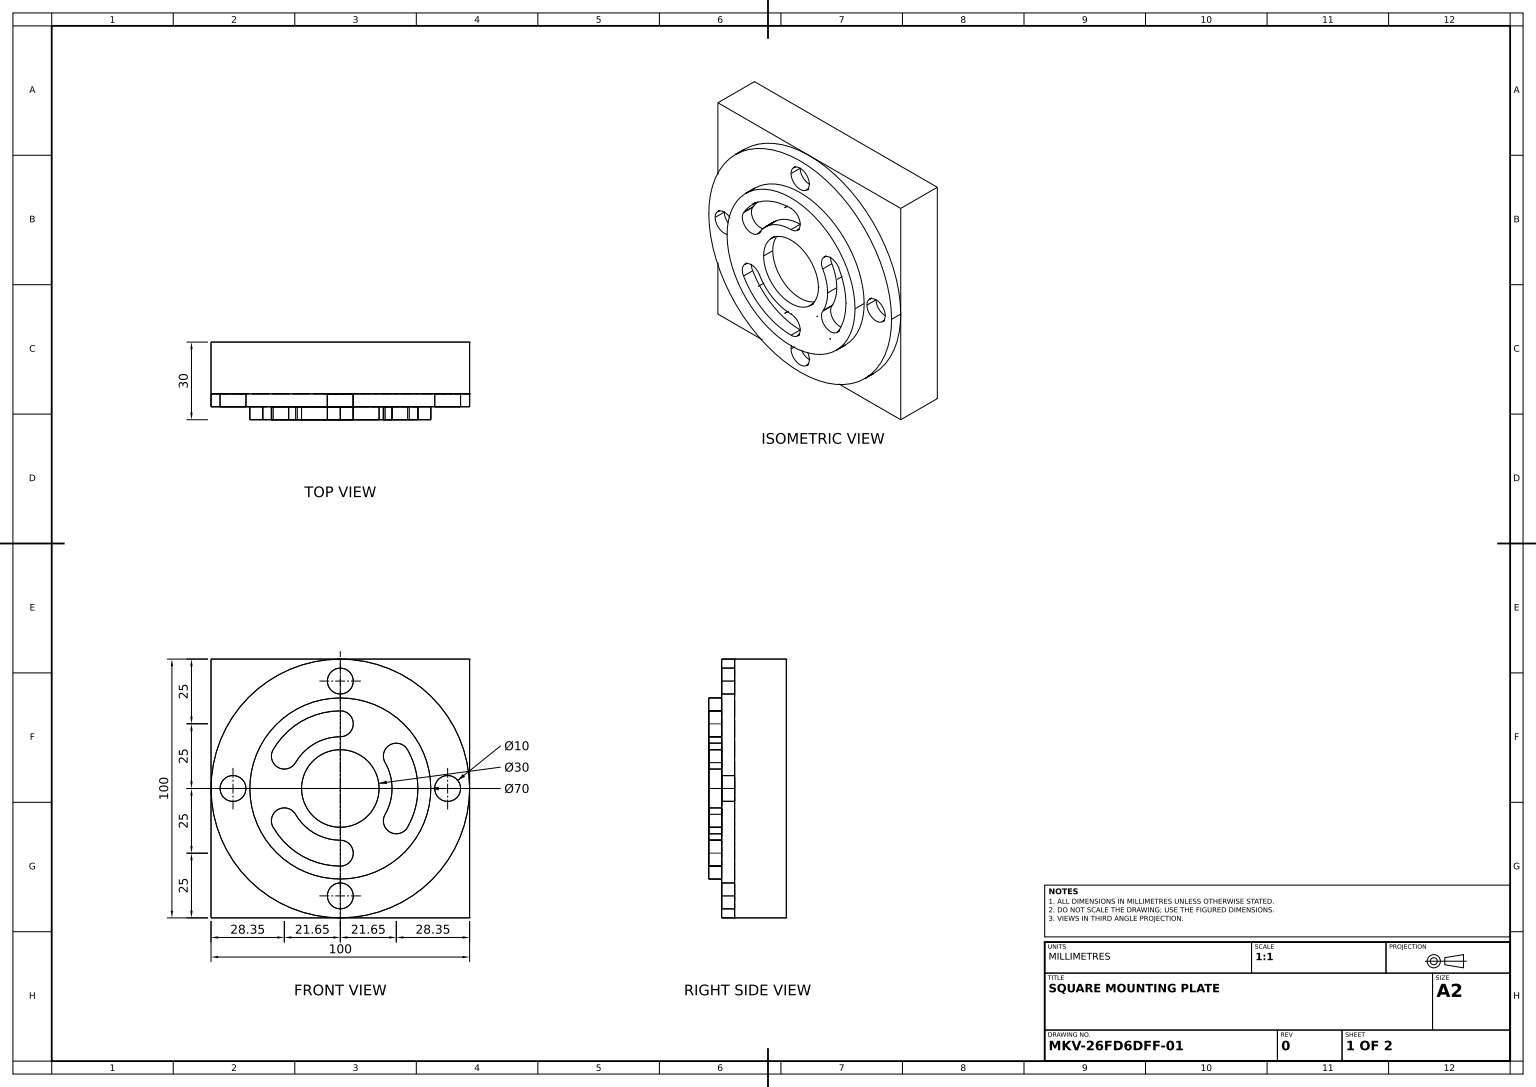
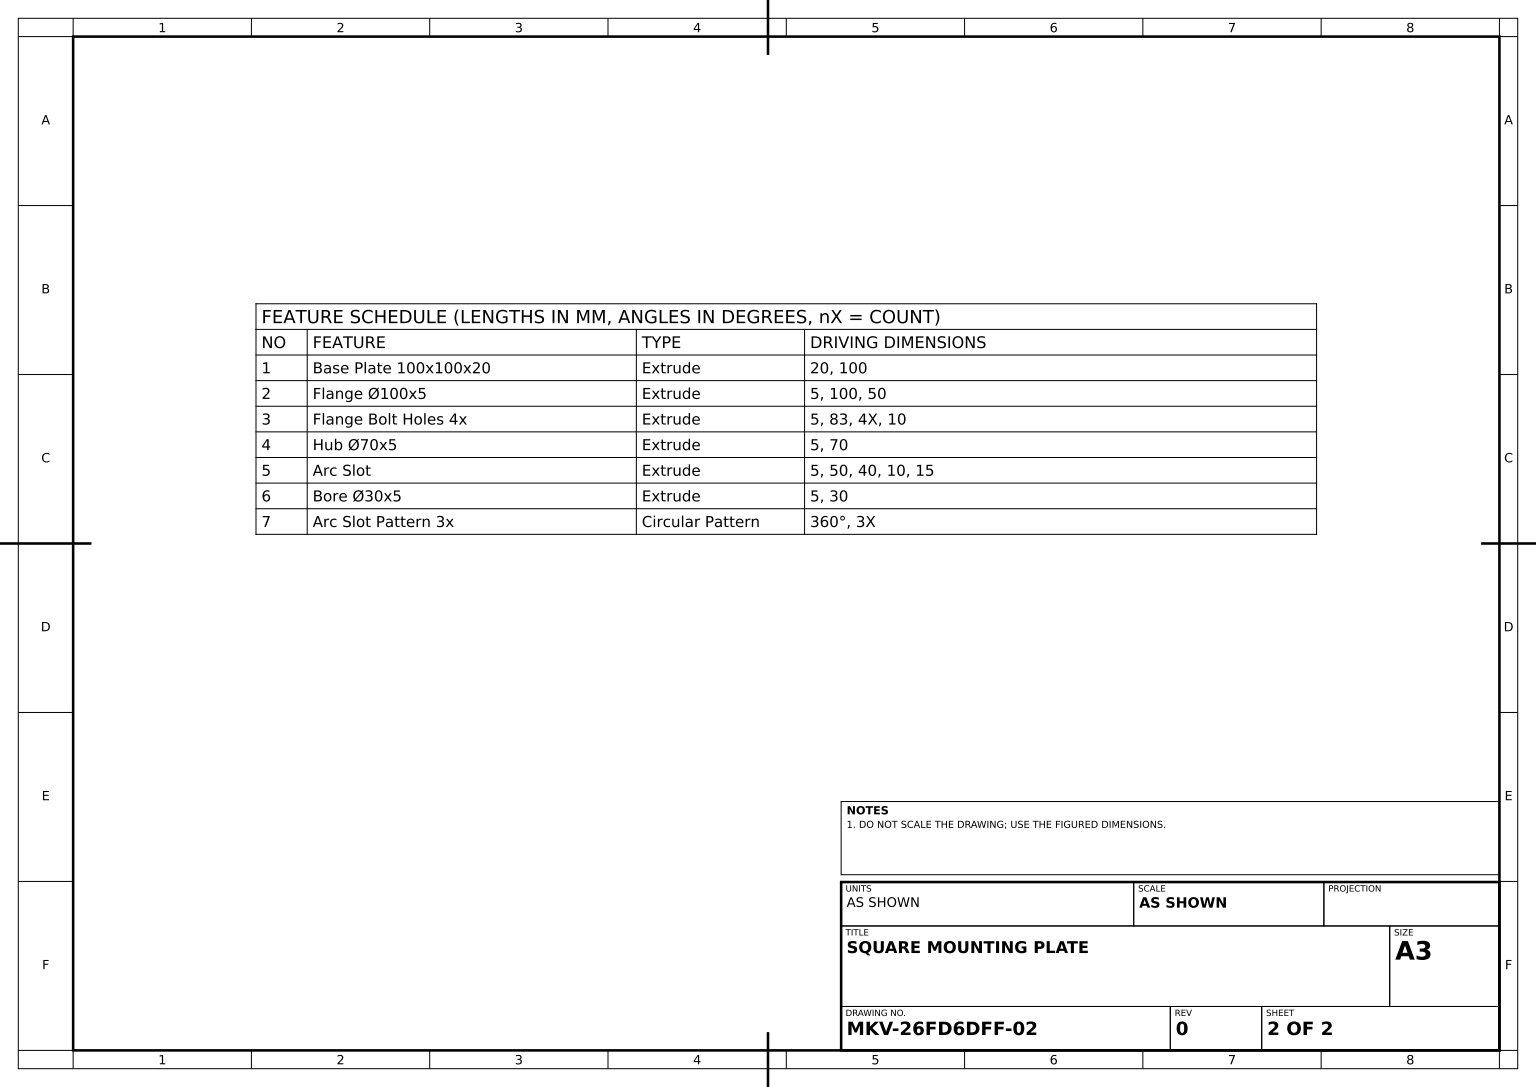
SolidWorks part; units mm, degrees
material "Plain Carbon Steel"
ref_plane "Front Plane" through (0, 0, 0) normal (0, 0, 1) x (1, 0, 0)
ref_plane "Top Plane" through (0, 0, 0) normal (0, 1, 0) x (1, 0, 0)
ref_plane "Right Plane" through (0, 0, 0) normal (1, 0, 0) x (0, 0, -1)
sketch "Base Plate Sketch" plane through (0, 0, 0) normal (0, 0, 1) x (1, 0, 0)
  line L0 (0, 0) -> (100, 0)
  line L1 (100, 0) -> (100, 100)
  line L2 (100, 100) -> (0, 100)
  line L3 (0, 100) -> (0, 0)
  dimension "D1" = 100
  dimension "D2" = 100
extrude "Base Plate 100x100x20" add sketch "Base Plate Sketch" along normal blind 20
sketch "Flange Sketch" plane through (0, 0, 20) normal (0, 0, 1) x (1, 0, 0)
  line L0 (0, 100) -> (0, 0) construction
  line L1 (0, 0) -> (100, 0) construction
  circle A0 centre (50, 50) radius 50
  dimension "D1" = 100
  dimension "D2" = 50
  dimension "D3" = 50
extrude "Flange Ø100x5" add sketch "Flange Sketch" along normal blind 5
sketch "Flange Bolt Holes Sketch" plane through (0, 0, 25) normal (0, 0, 1) x (1, 0, 0)
  line L0 (50, 50) -> (50, 91.5) construction
  line L1 (50, 50) -> (50, 8.5) construction
  line L2 (50, 50) -> (91.5, 50) construction
  line L3 (50, 50) -> (8.5, 50) construction
  circle A0 centre (50, 50) radius 41.5 construction
  circle A1 centre (50, 91.5) radius 5
  circle A2 centre (91.5, 50) radius 5
  circle A3 centre (50, 8.5) radius 5
  circle A4 centre (8.5, 50) radius 5
  dimension "D1" = 83
  dimension "D2" = 4
  dimension "D3" = 10
extrude "Flange Bolt Holes 4x" cut sketch "Flange Bolt Holes Sketch" against normal blind 5
sketch "Hub Sketch" plane through (0, 0, 25) normal (0, 0, 1) x (1, 0, 0)
  circle A0 centre (50, 50) radius 35
  dimension "D1" = 70
extrude "Hub Ø70x5" add sketch "Hub Sketch" along normal blind 5
sketch "Arc Slot Sketch" plane through (0, 0, 30) normal (0, 0, 1) x (1, 0, 0)
  line L0 (50, 50) -> (50, 100) construction
  line L1 (50, 50) -> (50, 0) construction
  line L2 (50, 50) -> (100, 50) construction
  line L3 (50, 50) -> (0, 50) construction
  circle A1 centre (50, 50) radius 25 construction
  arc A2 (50, 70) -> (32.6795, 60) centre (50, 50) ccw
  circle A3 centre (50, 50) radius 50 construction
  arc A4 (50, 70) -> (50, 80) centre (50, 75) ccw
  arc A5 (24.0192, 65) -> (32.6795, 60) centre (28.3494, 62.5) ccw
  arc A6 (50, 80) -> (24.0192, 65) centre (50, 50) ccw
  dimension "D2" = 50
  dimension "D3" = 40
  dimension "D4" = 10
  dimension "D5" = 10
  dimension "D6" = 15
extrude "Arc Slot" cut sketch "Arc Slot Sketch" against normal blind 5
sketch "Bore Sketch" plane through (0, 0, 30) normal (0, 0, 1) x (1, 0, 0)
  circle A0 centre (50, 50) radius 15
  dimension "D1" = 30
extrude "Bore Ø30x5" cut sketch "Bore Sketch" against normal blind 5
pattern_circular "Arc Slot Pattern 3x" count 3 over 360 about axis through (50, 50, 0) along (0, 0, 1) of "Arc Slot"
